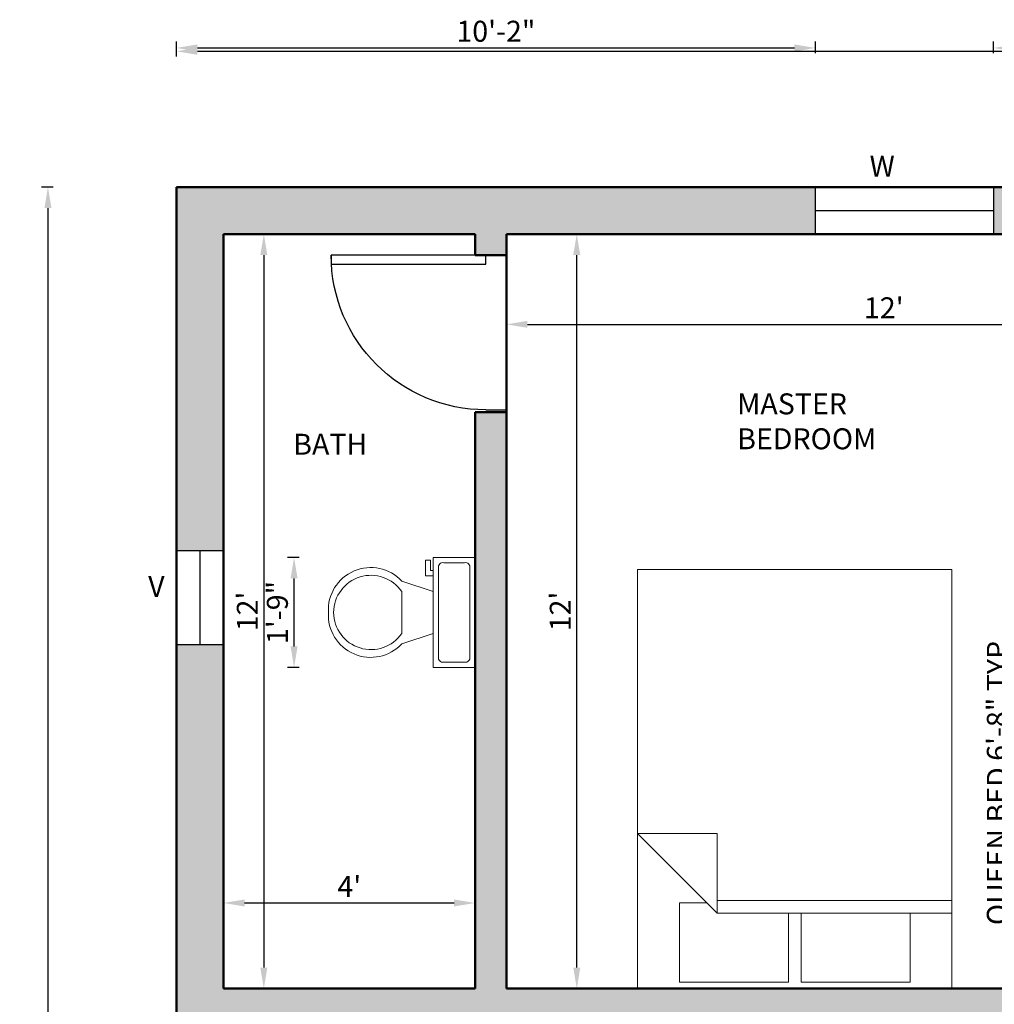
# Model space of a CAD drawing. Units: inches. Extents: x -31 to 511, y -453 to 49.
# Tile 2 of 4: x -29 to 157, y -142 to 46. Entities that reach past the tile are written whole.
import ezdxf

# ---------------------------------------------------------------- set-up
doc = ezdxf.new("R2010")
doc.units = ezdxf.units.IN
for name, color, linetype, lineweight in [('A-ANNO-DIMS', 2, 'Continuous', 18), ('A-ANNO-TEXT', 7, 'Continuous', 18), ('A-AREA-IDEN', 7, 'Continuous', 25), ('A-DOOR', 3, 'Continuous', 25), ('A-FLOR-FIXT', 9, 'Continuous', 18), ('A-FURN', 8, 'Continuous', 18), ('A-GLAZ', 4, 'Continuous', 25), ('A-WALL', 7, 'Continuous', 50), ('A-WALL-PATT', 252, 'Continuous', 13)]:
    doc.layers.add(name, color=color, linetype=linetype, lineweight=lineweight)
doc.styles.get("Standard").update_dxf_attribs({"font": 'arial.ttf'})
doc.dimstyles.new('ISO-25', dxfattribs={"dimtxt": 4, "dimasz": 4, "dimexe": 1.25, "dimexo": 0.625, "dimtad": 1, "dimlunit": 3, "dimtxsty": 'Standard', "dimcen": 2.5, "dimadec": 0, "dimazin": 0, "dimtfac": 1, "dimtmove": 0, "dimatfit": 3, "dimfxl": 1, "dimfxlon": 1, "dimarcsym": 0})

# ---------------------------------------------------------------- blocks, each defined once
blk = doc.blocks.new('*U2')
for p, q in [((0, 0), (0, -100)), ((750, 0), (750, -100))]:
    blk.add_line(p, q)
blk.add_lwpolyline([(0, 0), (0, 750), (43.75, 750), (43.75, 0)], close=True)
blk.add_arc((0, 0), 750, 0, 90)
blk = doc.blocks.new('*U4')
for p, q in [((9.5, -6), (9.5, -2)), ((-10, -8.5), (-8, -8.5)), ((-10, -9.5), (-10, -8.5)), ((-8, -8.5), (-8, -8)), ((-7, -8), (-7, -9.5)), ((-4, -8), (-6, -14)), ((4, -8), (6, -14)), ((-7, -9.5), (-10, -9.5)), ((4, -14), (-4, -14))]:
    blk.add_line(p, q)
blk.add_lwpolyline([(10.5, -8), (10.5, 0), (-10.5, 0), (-10.5, -8)], close=True)
for points in [[(8.5, -1), (-8.5, -1)], [(-9.5, -2), (-9.5, -6)], [(-8.5, -7), (8.5, -7)]]:
    blk.add_lwpolyline(points)
for centre, radius, start, end in [((-8.625, -1.875), 0.8839, 81.8699, 188.1301), ((8.625, -1.875), 0.8839, 351.8699, 98.1301), ((-8.625, -6.125), 0.8839, 171.869898, 278.1301), ((8.625, -6.125), 0.8839, 261.8699, 8.1301), ((-0.4772, -19.9188), 8.0953, 133.01722, 273.38), ((0.0374, -19.8731), 7.127, 124.50543, 269.7), ((-0.0373, -19.8731), 7.127, 270.3, 55.4946), ((0.4773, -19.9188), 8.0953, 266.62, 46.9828)]:
    blk.add_arc(centre, radius, start, end)
blk = doc.blocks.new('Bed - Queen')
for p, q in [((0, -80.00003), (0, 0)), ((0, 0), (59.99999, 0)), ((59.99999, 0), (59.99999, -80.00003)), ((7.99999, -1.2), (28.79998, -1.2)), ((7.99999, -14.4), (7.99999, -1.2)), ((28.79998, -1.2), (28.79998, -14.4)), ((31.19999, -1.2), (51.99999, -1.2)), ((31.19999, -14.4), (31.19999, -1.2)), ((51.99999, -1.2), (51.99999, -16.4)), ((0, -14.4), (44.8, -14.4)), ((59.99999, -29.6), (44.8, -14.4)), ((44.8, -14.4), (44.8, -29.6)), ((44.8, -16.8), (0, -16.8)), ((51.99999, -16.4), (46.79936, -16.4)), ((44.8, -29.6), (59.99999, -29.6)), ((59.99999, -80.00003), (0, -80.00003))]:
    blk.add_line(p, q)
blk = doc.blocks.new('*D12')
at = {"layer": 'A-ANNO-DIMS', "color": 0, "lineweight": -2, "transparency": 16777216}
for p, q in [((16.15, 4.62), (18.4, 4.62)), ((17.15, 0.62), (17.15, -135.38)), ((16.15, -139.38), (18.4, -139.38))]:
    blk.add_line(p, q, dxfattribs=at)
at = {"layer": 'A-ANNO-DIMS', "color": 0, "transparency": 16777216}
for points in [[(16.48, 0.62), (17.82, 0.62), (17.15, 4.62)], [(16.48, -135.38), (17.82, -135.38), (17.15, -139.38)]]:
    blk.add_solid(points, dxfattribs=at)
at = {"layer": 'Defpoints', "color": 0, "transparency": 16777216}
for p in [(9.46, 4.62), (9.46, -139.38), (17.15, -139.38)]:
    blk.add_point(p, dxfattribs=at)
at = {"layer": 'A-ANNO-DIMS', "color": 0, "transparency": 16777216, "insert": (14.52, -67.38), "char_height": 4, "attachment_point": 5, "rotation": 90}
blk.add_mtext("12'", dxfattribs=at)
blk = doc.blocks.new('*D13')
at = {"layer": 'A-ANNO-DIMS', "color": 0, "lineweight": -2, "transparency": 16777216}
for p, q in [((9.46, -124.04), (9.46, -121.79)), ((57.46, -124.04), (57.46, -121.79)), ((13.46, -123.04), (53.46, -123.04))]:
    blk.add_line(p, q, dxfattribs=at)
at = {"layer": 'A-ANNO-DIMS', "color": 0, "transparency": 16777216}
for points in [[(13.46, -122.37), (13.46, -123.7), (9.46, -123.04)], [(53.46, -122.37), (53.46, -123.7), (57.46, -123.04)]]:
    blk.add_solid(points, dxfattribs=at)
at = {"layer": 'Defpoints', "color": 0, "transparency": 16777216}
for p in [(57.46, -123.04), (9.46, -139.38), (57.46, -139.38)]:
    blk.add_point(p, dxfattribs=at)
at = {"layer": 'A-ANNO-DIMS', "color": 0, "transparency": 16777216, "insert": (33.46, -120.41), "char_height": 4, "attachment_point": 5}
blk.add_mtext("4'", dxfattribs=at)
blk = doc.blocks.new('*D14')
at = {"layer": 'A-ANNO-DIMS', "color": 0, "lineweight": -2, "transparency": 16777216}
for p, q in [((63.46, -11.59), (63.46, -13.84)), ((67.46, -12.59), (203.46, -12.59)), ((207.46, -11.59), (207.46, -13.84))]:
    blk.add_line(p, q, dxfattribs=at)
at = {"layer": 'A-ANNO-DIMS', "color": 0, "transparency": 16777216}
for points in [[(67.46, -11.92), (67.46, -13.25), (63.46, -12.59)], [(203.46, -11.92), (203.46, -13.25), (207.46, -12.59)]]:
    blk.add_solid(points, dxfattribs=at)
at = {"layer": 'Defpoints', "color": 0, "transparency": 16777216}
for p in [(63.46, 4.62), (207.46, 4.62), (207.46, -12.59)]:
    blk.add_point(p, dxfattribs=at)
at = {"layer": 'A-ANNO-DIMS', "color": 0, "transparency": 16777216, "insert": (135.46, -9.95), "char_height": 4, "attachment_point": 5}
blk.add_mtext("12'", dxfattribs=at)
blk = doc.blocks.new('*D15')
at = {"layer": 'A-ANNO-DIMS', "color": 0, "lineweight": -2, "transparency": 16777216}
for p, q in [((75.87, 4.62), (78.12, 4.62)), ((76.87, -135.38), (76.87, 0.62)), ((75.87, -139.38), (78.12, -139.38))]:
    blk.add_line(p, q, dxfattribs=at)
at = {"layer": 'A-ANNO-DIMS', "color": 0, "transparency": 16777216}
for points in [[(76.2, 0.62), (77.54, 0.62), (76.87, 4.62)], [(76.2, -135.38), (77.54, -135.38), (76.87, -139.38)]]:
    blk.add_solid(points, dxfattribs=at)
at = {"layer": 'Defpoints', "color": 0, "transparency": 16777216}
for p in [(63.46, 4.62), (76.87, 4.62), (63.46, -139.38)]:
    blk.add_point(p, dxfattribs=at)
at = {"layer": 'A-ANNO-DIMS', "color": 0, "transparency": 16777216, "insert": (74.24, -67.38), "char_height": 4, "attachment_point": 5, "rotation": 90}
blk.add_mtext("12'", dxfattribs=at)
blk = doc.blocks.new('*D26')
at = {"layer": 'A-ANNO-DIMS', "color": 0, "lineweight": -2, "transparency": 16777216}
for p, q in [((0.46, 38.54), (0.46, 40.79)), ((4.46, 39.54), (428.46, 39.54)), ((432.46, 38.54), (432.46, 40.79))]:
    blk.add_line(p, q, dxfattribs=at)
at = {"layer": 'A-ANNO-DIMS', "color": 0, "transparency": 16777216}
for points in [[(4.46, 40.2), (4.46, 38.87), (0.46, 39.54)], [(428.46, 40.2), (428.46, 38.87), (432.46, 39.54)]]:
    blk.add_solid(points, dxfattribs=at)
at = {"layer": 'Defpoints', "color": 0, "transparency": 16777216}
for p in [(432.46, 39.54), (0.46, 13.62), (432.46, 13.62)]:
    blk.add_point(p, dxfattribs=at)
at = {"layer": 'A-ANNO-DIMS', "color": 0, "transparency": 16777216, "insert": (216.46, 42.21), "char_height": 4, "attachment_point": 5}
blk.add_mtext("36'", dxfattribs=at)
blk = doc.blocks.new('*D27')
at = {"layer": 'A-ANNO-DIMS', "color": 0, "lineweight": -2, "transparency": 16777216}
for p, q in [((-23.05, 13.62), (-25.3, 13.62)), ((-24.05, 9.62), (-24.05, -414.38)), ((-23.05, -418.38), (-25.3, -418.38))]:
    blk.add_line(p, q, dxfattribs=at)
at = {"layer": 'A-ANNO-DIMS', "color": 0, "transparency": 16777216}
for points in [[(-24.71, 9.62), (-23.38, 9.62), (-24.05, 13.62)], [(-24.71, -414.38), (-23.38, -414.38), (-24.05, -418.38)]]:
    blk.add_solid(points, dxfattribs=at)
at = {"layer": 'Defpoints', "color": 0, "transparency": 16777216}
for p in [(0.46, 13.62), (-24.05, -418.38), (0.46, -418.38)]:
    blk.add_point(p, dxfattribs=at)
at = {"layer": 'A-ANNO-DIMS', "color": 0, "transparency": 16777216, "insert": (-26.72, -202.38), "char_height": 4, "attachment_point": 5, "rotation": 90}
blk.add_mtext("36'", dxfattribs=at)
blk = doc.blocks.new('WIN-34IN')
blk.add_line((0, 4.5), (34, 4.5))
blk.add_lwpolyline([(0, 9), (34, 9), (34, 0), (0, 0)], close=True)
blk = doc.blocks.new('VENT-18IN')
blk.add_line((4.5, 18), (4.5, 0))
blk.add_lwpolyline([(0, 18), (9, 18), (9, 0), (0, 0)], close=True)
blk = doc.blocks.new('*D34')
at = {"layer": 'A-ANNO-DIMS', "color": 0, "lineweight": -2, "transparency": 16777216}
for p, q in [((159.47, -59.38), (161.72, -59.38)), ((160.47, -63.38), (160.47, -135.38)), ((159.47, -139.38), (161.72, -139.38))]:
    blk.add_line(p, q, dxfattribs=at)
at = {"layer": 'A-ANNO-DIMS', "color": 0, "transparency": 16777216}
for points in [[(159.8, -63.38), (161.13, -63.38), (160.47, -59.38)], [(159.8, -135.38), (161.13, -135.38), (160.47, -139.38)]]:
    blk.add_solid(points, dxfattribs=at)
at = {"layer": 'Defpoints', "color": 0, "transparency": 16777216}
for p in [(148.47, -59.38), (148.47, -139.38), (160.47, -139.38)]:
    blk.add_point(p, dxfattribs=at)
at = {"layer": 'A-ANNO-DIMS', "color": 0, "transparency": 16777216, "insert": (157.65, -99.38), "char_height": 4, "attachment_point": 5, "rotation": 90}
blk.add_mtext('QUEEN BED 6\'-8" TYP.', dxfattribs=at)
blk = doc.blocks.new('*D35')
at = {"layer": 'A-ANNO-DIMS', "color": 0, "lineweight": -2, "transparency": 16777216}
for p, q in [((88.47, -150.38), (88.47, -152.63)), ((144.47, -151.38), (92.47, -151.38)), ((148.47, -150.38), (148.47, -152.63))]:
    blk.add_line(p, q, dxfattribs=at)
at = {"layer": 'A-ANNO-DIMS', "color": 0, "transparency": 16777216}
for points in [[(92.47, -150.71), (92.47, -152.05), (88.47, -151.38)], [(144.47, -150.71), (144.47, -152.05), (148.47, -151.38)]]:
    blk.add_solid(points, dxfattribs=at)
at = {"layer": 'Defpoints', "color": 0, "transparency": 16777216}
for p in [(88.47, -139.38), (148.47, -139.38), (88.47, -151.38)]:
    blk.add_point(p, dxfattribs=at)
at = {"layer": 'A-ANNO-DIMS', "color": 0, "transparency": 16777216, "insert": (118.47, -148.71), "char_height": 4, "attachment_point": 5}
blk.add_mtext('5\'-0" TYP.', dxfattribs=at)
blk = doc.blocks.new('*D51')
at = {"layer": 'A-ANNO-DIMS', "color": 0, "lineweight": -2, "transparency": 16777216}
for p, q in [((508.55, 0.62), (510.8, 0.62)), ((509.55, -3.38), (509.55, -25.38)), ((508.55, -29.38), (510.8, -29.38))]:
    blk.add_line(p, q, dxfattribs=at)
at = {"layer": 'A-ANNO-DIMS', "color": 0, "transparency": 16777216}
for points in [[(508.88, -3.38), (510.22, -3.38), (509.55, 0.62)], [(508.88, -25.38), (510.22, -25.38), (509.55, -29.38)]]:
    blk.add_solid(points, dxfattribs=at)
at = {"layer": 'Defpoints', "color": 0, "transparency": 16777216}
for p in [(57.46, 0.62), (57.46, -29.38), (509.55, -29.38)]:
    blk.add_point(p, dxfattribs=at)
at = {"layer": 'A-ANNO-DIMS', "color": 0, "transparency": 16777216, "insert": (506.88, -14.38), "char_height": 4, "attachment_point": 5, "rotation": 90}
blk.add_mtext('2\'-6"', dxfattribs=at)
blk = doc.blocks.new('*D54')
at = {"layer": 'A-ANNO-DIMS', "color": 0, "lineweight": -2, "transparency": 16777216}
for p, q in [((0.46, 39.17), (0.46, 41.42)), ((122.41, 39.17), (122.41, 41.42)), ((4.46, 40.17), (118.41, 40.17))]:
    blk.add_line(p, q, dxfattribs=at)
at = {"layer": 'A-ANNO-DIMS', "color": 0, "transparency": 16777216}
for points in [[(4.46, 40.84), (4.46, 39.5), (0.46, 40.17)], [(118.41, 40.84), (118.41, 39.5), (122.41, 40.17)]]:
    blk.add_solid(points, dxfattribs=at)
at = {"layer": 'Defpoints', "color": 0, "transparency": 16777216}
for p in [(122.41, 40.17), (0.46, 13.62), (122.41, 13.62)]:
    blk.add_point(p, dxfattribs=at)
at = {"layer": 'A-ANNO-DIMS', "color": 0, "transparency": 16777216, "insert": (61.44, 42.84), "char_height": 4, "attachment_point": 5}
blk.add_mtext('10\'-2"', dxfattribs=at)
blk = doc.blocks.new('*D55')
at = {"layer": 'A-ANNO-DIMS', "color": 0, "lineweight": -2, "transparency": 16777216}
for p, q in [((156.41, 39.17), (156.41, 41.42)), ((267.57, 39.17), (267.57, 41.42)), ((160.41, 40.17), (263.57, 40.17))]:
    blk.add_line(p, q, dxfattribs=at)
at = {"layer": 'A-ANNO-DIMS', "color": 0, "transparency": 16777216}
for points in [[(160.41, 40.84), (160.41, 39.5), (156.41, 40.17)], [(263.57, 40.84), (263.57, 39.5), (267.57, 40.17)]]:
    blk.add_solid(points, dxfattribs=at)
at = {"layer": 'Defpoints', "color": 0, "transparency": 16777216}
for p in [(267.57, 40.17), (156.41, 13.62), (267.57, 13.62)]:
    blk.add_point(p, dxfattribs=at)
at = {"layer": 'A-ANNO-DIMS', "color": 0, "transparency": 16777216, "insert": (211.99, 42.84), "char_height": 4, "attachment_point": 5}
blk.add_mtext('9\'-3"', dxfattribs=at)
blk = doc.blocks.new('*D65')
at = {"layer": 'A-ANNO-DIMS', "color": 0, "lineweight": -2, "transparency": 16777216}
for p, q in [((29.47, -443.93), (29.47, -446.18)), ((33.47, -444.93), (53.47, -444.93)), ((57.47, -443.93), (57.47, -446.18))]:
    blk.add_line(p, q, dxfattribs=at)
at = {"layer": 'A-ANNO-DIMS', "color": 0, "transparency": 16777216}
for points in [[(33.47, -444.26), (33.47, -445.6), (29.47, -444.93)], [(53.47, -444.26), (53.47, -445.6), (57.47, -444.93)]]:
    blk.add_solid(points, dxfattribs=at)
at = {"layer": 'Defpoints', "color": 0, "transparency": 16777216}
for p in [(29.47, -67.58), (57.47, -78.08), (57.47, -444.93)]:
    blk.add_point(p, dxfattribs=at)
at = {"layer": 'A-ANNO-DIMS', "color": 0, "transparency": 16777216, "insert": (43.47, -442.3), "char_height": 4, "attachment_point": 5}
blk.add_mtext('2\'-4"', dxfattribs=at)
blk = doc.blocks.new('*D66')
at = {"layer": 'A-ANNO-DIMS', "color": 0, "lineweight": -2, "transparency": 16777216}
for p, q in [((23.92, -57.08), (21.67, -57.08)), ((22.92, -74.08), (22.92, -61.08)), ((23.92, -78.08), (21.67, -78.08))]:
    blk.add_line(p, q, dxfattribs=at)
at = {"layer": 'A-ANNO-DIMS', "color": 0, "transparency": 16777216}
for points in [[(22.26, -61.08), (23.59, -61.08), (22.92, -57.08)], [(22.26, -74.08), (23.59, -74.08), (22.92, -78.08)]]:
    blk.add_solid(points, dxfattribs=at)
at = {"layer": 'Defpoints', "color": 0, "transparency": 16777216}
for p in [(22.92, -57.08), (49.47, -57.08), (49.47, -78.08)]:
    blk.add_point(p, dxfattribs=at)
at = {"layer": 'A-ANNO-DIMS', "color": 0, "transparency": 16777216, "insert": (20.25, -67.58), "char_height": 4, "attachment_point": 5, "rotation": 90}
blk.add_mtext('1\'-9"', dxfattribs=at)
blk = doc.blocks.new('*D72')
at = {"layer": 'A-ANNO-DIMS', "color": 0, "lineweight": -2, "transparency": 16777216}
for p, q in [((509.55, 8.62), (509.55, 12.62)), ((508.55, 4.62), (510.8, 4.62)), ((509.55, 4.62), (509.55, 0.62)), ((508.55, 0.62), (510.8, 0.62)), ((509.55, -3.38), (509.55, -19.26))]:
    blk.add_line(p, q, dxfattribs=at)
at = {"layer": 'A-ANNO-DIMS', "color": 0, "transparency": 16777216}
for points in [[(508.88, 8.62), (510.22, 8.62), (509.55, 4.62)], [(508.88, -3.38), (510.22, -3.38), (509.55, 0.62)]]:
    blk.add_solid(points, dxfattribs=at)
at = {"layer": 'Defpoints', "color": 0, "transparency": 16777216}
for p in [(57.46, 4.62), (57.46, 0.62), (509.55, 0.62)]:
    blk.add_point(p, dxfattribs=at)
at = {"layer": 'A-ANNO-DIMS', "color": 0, "transparency": 16777216, "insert": (506.88, -13.32), "char_height": 4, "attachment_point": 5, "rotation": 90}
blk.add_mtext('0\'-4"', dxfattribs=at)

msp = doc.modelspace()

# ---------------------------------------------------------------- hatches: boundary and pattern name
at = {"layer": 'A-WALL-PATT'}
h = msp.add_hatch(color=256, dxfattribs=at)
h.dxf.hatch_style = 1
h.paths.add_polyline_path([(122.408, 13.62), (0.465, 13.62), (0.465, -55.742), (9.465, -55.742), (9.465, 4.62), (57.465, 4.62), (57.465, 0.62), (59.528, 0.62), (63.465, 0.62), (63.465, 4.62), (122.408, 4.62)])
h.paths.add_polyline_path([(267.569, 13.62), (156.408, 13.62), (156.408, 4.62), (207.465, 4.62), (207.465, -139.38), (203.465, -139.38), (203.465, -140.534), (203.465, -145.38), (217.465, -145.38), (217.465, -140.567), (217.465, -139.38), (213.465, -139.38), (213.465, 4.62), (267.569, 4.62)])
h.paths.add_polyline_path([(432.465, 13.62), (301.569, 13.62), (301.569, 4.62), (357.465, 4.62), (357.465, 0.312), (361.402, 0.312), (363.465, 0.312), (363.465, 4.62), (423.465, 4.62), (423.465, -55.742), (432.465, -55.742)])
h.paths.add_polyline_path([(432.465, -73.742), (423.465, -73.742), (423.465, -139.38), (363.465, -139.38), (363.465, -29.688), (357.465, -29.688), (357.465, -139.38), (253.542, -139.38, -0.0082235), (253.561, -140.567), (253.561, -145.38), (423.465, -145.38), (423.465, -409.38), (414.601, -409.38), (414.601, -412.759), (414.601, -418.38), (432.465, -418.38)])
h.paths.add_polyline_path([(167.12, -140.534, -0.00794), (167.139, -139.38), (63.465, -139.38), (63.465, -29.38), (57.465, -29.38), (57.465, -57.083), (57.472, -57.083), (57.472, -78.083), (57.465, -139.38), (9.465, -139.38), (9.465, -73.742), (0.465, -73.742), (0.465, -179.759), (9.465, -179.759), (9.465, -145.38), (167.12, -145.38)])
h.paths.add_polyline_path([(372.446, -412.759, -0.0200643), (372.581, -409.38), (327.465, -409.38), (327.465, -265.38), (285.454, -265.38), (285.454, -271.38), (321.465, -271.38), (321.465, -409.38), (273.096, -409.38), (273.096, -418.38), (372.446, -418.38)], flags=17)
h.paths.add_polyline_path([(239.096, -409.38), (189.465, -409.38), (189.465, -271.38), (243.454, -271.38), (243.454, -265.38), (183.465, -265.38), (183.465, -409.38), (156.552, -409.38), (156.552, -418.38), (239.096, -418.38)])
h.paths.add_polyline_path([(122.552, -409.38), (111.465, -409.38), (111.465, -325.38), (105.465, -325.38), (105.465, -409.38), (72.938, -409.38), (72.938, -418.38), (122.552, -418.38)])
h.paths.add_polyline_path([(38.938, -409.38), (9.465, -409.38), (9.465, -341.741), (0.465, -341.741), (0.465, -418.38), (38.938, -418.38)])
h.paths.add_polyline_path([(9.465, -213.759), (0.465, -213.759), (0.465, -307.741), (9.465, -307.741)])

# ---------------------------------------------------------------- linework, layer by layer
at = {"layer": 'A-WALL'}
for p, q in [((0.465, 13.62), (432.465, 13.62)), ((0.465, -418.38), (0.465, 13.62)), ((9.465, 4.62), (57.465, 4.62)), ((9.465, -139.38), (9.465, 4.62)), ((57.465, 0.62), (57.465, 4.62)), ((63.465, 4.62), (207.465, 4.62)), ((63.465, -139.38), (63.465, 4.62)), ((63.465, 0.62), (57.465, 0.62)), ((57.465, -139.38), (57.465, -29.38)), ((63.465, -29.38), (57.465, -29.38)), ((9.465, -139.38), (57.465, -139.38)), ((63.465, -139.38), (167.465, -139.38))]:
    msp.add_line(p, q, dxfattribs=at)

# ---------------------------------------------------------------- block references
at = {"layer": 'A-DOOR', "xscale": -0.0393700787401575, "yscale": 0.0393700787401575, "zscale": 0.0393700787401575, "rotation": 90}
msp.add_blockref('*U2', (59.528, 0.62), dxfattribs=at)
at = {"layer": 'A-FLOR-FIXT', "rotation": 270}
msp.add_blockref('*U4', (57.472, -67.583), dxfattribs=at)
at = {"layer": 'A-FURN', "rotation": 180}
msp.add_blockref('Bed - Queen', (148.466, -139.38), dxfattribs=at)
at = {"layer": 'A-GLAZ'}
for name, p in [('WIN-34IN', (122.408, 4.62)), ('VENT-18IN', (0.465, -73.742))]:
    msp.add_blockref(name, p, dxfattribs=at)

# ---------------------------------------------------------------- texts
at = {"layer": 'A-ANNO-TEXT', "char_height": 4, "attachment_point": 1}
for s, width, insert in [('W', 12.06723, (132.756, 19.584)), ('V', 7.25664, (-4.927, -60.604))]:
    msp.add_mtext_dynamic_manual_height_columns(s, width=width, gutter_width=12.5, heights=[0], dxfattribs=dict(at, insert=insert))
at = {"layer": 'A-AREA-IDEN', "char_height": 4, "attachment_point": 1}
for s, width, insert in [('MASTER\\PBEDROOM', 56.19275, (107.481, -25.767)), ('BATH', 26.07232, (22.754, -33.473))]:
    msp.add_mtext_dynamic_manual_height_columns(s, width=width, gutter_width=12.5, heights=[0], dxfattribs=dict(at, insert=insert))

# ---------------------------------------------------------------- dimensions: what is measured, and where the dimension line sits
at = {"layer": 'A-ANNO-DIMS'}
for base, p1, p2, angle, override, picture, middle in [((122.408, 40.17), (0.465, 13.62), (122.408, 13.62), 0, {"dimdec": 1, "dimlfac": 1, "dimrnd": 0, "dimzin": 1, "dimdsep": 46, "dimlunit": 4, "dimfrac": 2}, '*D54', (61.436, 42.838)), ((-24.047, -418.38), (0.465, 13.62), (0.465, -418.38), 90, {"dimclrd": 0, "dimclre": 0, "dimclrt": 0}, '*D27', (-26.716, -202.38)), ((509.551, 0.62), (57.465, 4.62), (57.465, 0.62), 90, {"dimdec": 1, "dimlfac": 1, "dimrnd": 0, "dimzin": 1, "dimdsep": 46, "dimlunit": 4, "dimfrac": 2}, '*D72', (506.883, -13.321)), ((17.149, -139.38), (9.465, 4.62), (9.465, -139.38), 90, {"dimclrd": 0, "dimclre": 0, "dimclrt": 0}, '*D12', (14.516, -67.38)), ((76.87, 4.62), (63.465, -139.38), (63.465, 4.62), 90, {"dimclrd": 0, "dimclre": 0, "dimclrt": 0}, '*D15', (74.237, -67.38)), ((509.551, -29.38), (57.465, 0.62), (57.465, -29.38), 90, {"dimdec": 1, "dimlfac": 1, "dimrnd": 0, "dimzin": 1, "dimdsep": 46, "dimlunit": 4, "dimfrac": 2}, '*D51', (506.883, -14.38)), ((22.922, -57.083), (49.472, -78.083), (49.472, -57.083), 90, {"dimdec": 1, "dimlfac": 1, "dimrnd": 0, "dimzin": 1, "dimdsep": 46, "dimlunit": 4, "dimfrac": 2}, '*D66', (20.255, -67.583))]:
    dim = msp.add_linear_dim(base=base, p1=p1, p2=p2, angle=angle, dimstyle='ISO-25', override=override, dxfattribs=at)
    dim.commit()
    dim.dimension.update_dxf_attribs({"geometry": picture, "text_midpoint": middle})
for base, p1, p2, override, picture, middle in [((267.569, 40.17), (156.408, 13.62), (267.569, 13.62), {"dimdec": 1, "dimlfac": 1, "dimrnd": 0, "dimzin": 1, "dimdsep": 46, "dimlunit": 4, "dimfrac": 2}, '*D55', (211.988, 42.839)), ((432.465, 39.538), (0.465, 13.62), (432.465, 13.62), {"dimclrd": 0, "dimclre": 0, "dimclrt": 0}, '*D26', (216.465, 42.207)), ((207.465, -12.586), (63.465, 4.62), (207.465, 4.62), {"dimclrd": 0, "dimclre": 0, "dimclrt": 0}, '*D14', (135.465, -9.952)), ((57.472, -444.93), (29.472, -67.583), (57.472, -78.083), {"dimdec": 1, "dimlfac": 1, "dimrnd": 0, "dimzin": 1, "dimdsep": 46, "dimlunit": 4, "dimfrac": 2}, '*D65', (43.472, -442.297)), ((57.465, -123.035), (9.465, -139.38), (57.465, -139.38), {"dimclrd": 0, "dimclre": 0, "dimclrt": 0}, '*D13', (33.465, -120.41))]:
    dim = msp.add_linear_dim(base=base, p1=p1, p2=p2, dimstyle='ISO-25', override=override, dxfattribs=at)
    dim.commit()
    dim.dimension.update_dxf_attribs({"geometry": picture, "text_midpoint": middle})
for base, p1, p2, angle, text, picture, middle in [((160.466, -139.38), (148.466, -59.38), (148.466, -139.38), 270, 'QUEEN BED <> TYP.', '*D34', (157.65, -99.38)), ((88.466, -151.38), (148.466, -139.38), (88.466, -139.38), 180, '<> TYP.', '*D35', (118.466, -148.712))]:
    dim = msp.add_linear_dim(base=base, p1=p1, p2=p2, angle=angle, text=text, dimstyle='ISO-25', override={"dimdec": 1, "dimlfac": 1, "dimrnd": 0, "dimzin": 1, "dimdsep": 46, "dimlunit": 4, "dimfrac": 2}, dxfattribs=at)
    dim.commit()
    dim.dimension.update_dxf_attribs({"geometry": picture, "text_midpoint": middle})

doc.saveas('drawing.dxf')
